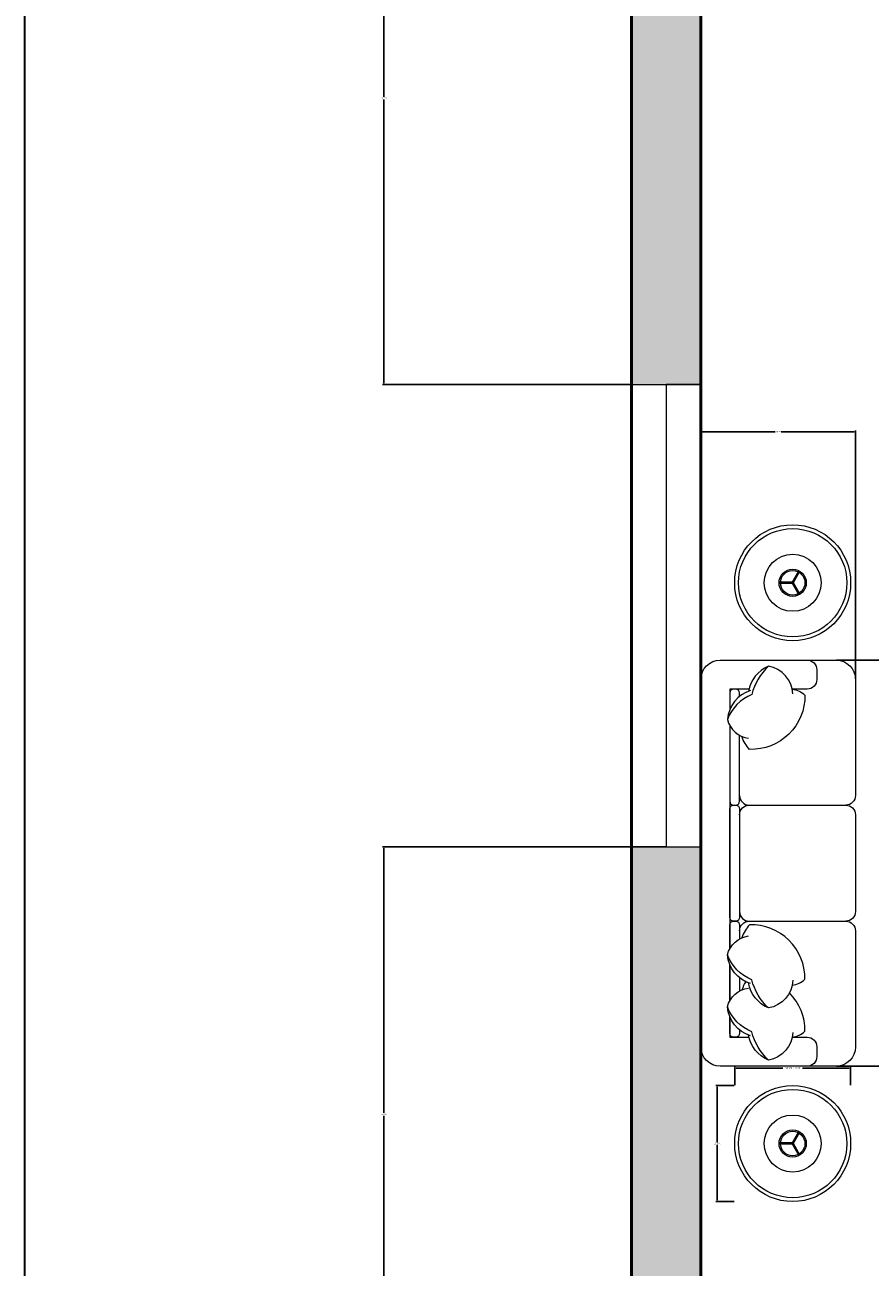
# Model space of a CAD drawing. Units: inches. Extents: x 1676 to 2199, y 1657 to 2783.
# Tile 2 of 10: x 1676 to 1786, y 1905 to 2066. Entities that reach past the tile are written whole.
import ezdxf

# ---------------------------------------------------------------- set-up
doc = ezdxf.new("R2010")
doc.units = ezdxf.units.IN
for name, color, linetype, lineweight in [('A-ANNO-DIMS', 2, 'Continuous', 18), ('A-ANNO-TTLB', 7, 'Continuous', 35), ('A-FURN', 8, 'Continuous', 13), ('A-GLAZ', 4, 'Continuous', 18), ('A-WALL', 7, 'Continuous', 50)]:
    doc.layers.add(name, color=color, linetype=linetype, lineweight=lineweight)
doc.layers.add('A-WALL-PATT', color=251, linetype='Continuous', lineweight=13, true_color=0x636466)
doc.styles.get("Standard").update_dxf_attribs({"font": 'arial.ttf'})
doc.dimstyles.get("Standard").update_dxf_attribs({"dimtxt": 0.18, "dimasz": 0.18, "dimexe": 0.18, "dimexo": 0.0625, "dimgap": 0.09, "dimtad": 0, "dimtih": 1, "dimtoh": 1, "dimdec": 4, "dimzin": 0, "dimdsep": 46, "dimtxsty": 'Standard', "dimcen": 0.09, "dimadec": 0, "dimazin": 0, "dimtfac": 1, "dimtdec": 4, "dimtofl": 0, "dimtmove": 0, "dimatfit": 3, "dimfxl": 1, "dimtolj": 1, "dimtzin": 0, "dimarcsym": 0})

# ---------------------------------------------------------------- blocks, each defined once
blk = doc.blocks.new('TABLE-END-ROUND')
at = {"ltscale": 0.03}
for p, q in [((0, 0.08), (-1.77, 0.08)), ((-0.07, 0.04), (0.82, 1.57)), ((0.07, -0.04), (0.95, 1.49)), ((0.07, 0.04), (0.95, -1.49)), ((0, -0.08), (-1.77, -0.08)), ((-0.07, -0.04), (0.82, -1.57))]:
    blk.add_line(p, q, dxfattribs=at)
for radius in [7.53, 3.7, 1.77, 1.59]:
    blk.add_circle((0, 0), radius, dxfattribs=at)
blk.add_circle((0, 0), 7.03)
blk = doc.blocks.new('WIN-60')
for p, q in [((0, 0), (9, 0)), ((9, 0), (4.5, 0)), ((4.5, 0), (4.5, -60)), ((4.5, -60), (0, -60)), ((0, -60), (9, -60))]:
    blk.add_line(p, q)
blk = doc.blocks.new('*D15')
at = {"layer": 'A-ANNO-DIMS', "color": 0, "lineweight": -2, "transparency": 16777216}
for p, q in [((1768.47, 1928.63), (1768.47, 1931.01)), ((1768.65, 1930.83), (1774.74, 1930.83)), ((1783.35, 1930.83), (1777.26, 1930.83)), ((1783.53, 1928.63), (1783.53, 1931.01))]:
    blk.add_line(p, q, dxfattribs=at)
at = {"layer": 'A-ANNO-DIMS', "color": 0, "transparency": 16777216}
for points in [[(1768.65, 1930.86), (1768.65, 1930.8), (1768.47, 1930.83)], [(1783.35, 1930.86), (1783.35, 1930.8), (1783.53, 1930.83)]]:
    blk.add_solid(points, dxfattribs=at)
at = {"layer": 'Defpoints', "color": 0, "transparency": 16777216}
for p in [(1783.53, 1930.83), (1768.47, 1928.57), (1783.53, 1928.57)]:
    blk.add_point(p, dxfattribs=at)
at = {"layer": 'A-ANNO-DIMS', "color": 0, "transparency": 16777216, "insert": (1776, 1930.83), "char_height": 0.18, "attachment_point": 5}
blk.add_mtext('\\A1;END TABLE 15 TYP.', dxfattribs=at)
blk = doc.blocks.new('*D16')
at = {"layer": 'A-ANNO-DIMS', "color": 0, "lineweight": -2, "transparency": 16777216}
for p, q in [((1768.41, 1928.57), (1766.03, 1928.57)), ((1766.21, 1928.39), (1766.21, 1921.22)), ((1766.21, 1913.68), (1766.21, 1920.85)), ((1768.41, 1913.5), (1766.03, 1913.5))]:
    blk.add_line(p, q, dxfattribs=at)
at = {"layer": 'A-ANNO-DIMS', "color": 0, "transparency": 16777216}
for points in [[(1766.18, 1928.39), (1766.24, 1928.39), (1766.21, 1928.57)], [(1766.18, 1913.68), (1766.24, 1913.68), (1766.21, 1913.5)]]:
    blk.add_solid(points, dxfattribs=at)
at = {"layer": 'Defpoints', "color": 0, "transparency": 16777216}
for p in [(1766.21, 1928.57), (1768.47, 1928.57), (1768.47, 1913.5)]:
    blk.add_point(p, dxfattribs=at)
at = {"layer": 'A-ANNO-DIMS', "color": 0, "transparency": 16777216, "insert": (1766.21, 1921.04), "char_height": 0.18, "attachment_point": 5}
blk.add_mtext('\\A1;15 TYP.', dxfattribs=at)
blk = doc.blocks.new('*D25')
at = {"layer": 'A-ANNO-DIMS', "color": 0, "lineweight": -2, "transparency": 16777216}
for p, q in [((1755.01, 1959.57), (1722.74, 1959.57)), ((1722.92, 1959.39), (1722.92, 1925.01)), ((1722.92, 1890.27), (1722.92, 1924.65)), ((1755.01, 1890.09), (1722.74, 1890.09))]:
    blk.add_line(p, q, dxfattribs=at)
at = {"layer": 'A-ANNO-DIMS', "color": 0, "transparency": 16777216}
for points in [[(1722.89, 1959.39), (1722.95, 1959.39), (1722.92, 1959.57)], [(1722.89, 1890.27), (1722.95, 1890.27), (1722.92, 1890.09)]]:
    blk.add_solid(points, dxfattribs=at)
at = {"layer": 'Defpoints', "color": 0, "transparency": 16777216}
for p in [(1722.92, 1959.57), (1755.07, 1959.57), (1755.07, 1890.09)]:
    blk.add_point(p, dxfattribs=at)
at = {"layer": 'A-ANNO-DIMS', "color": 0, "transparency": 16777216, "insert": (1722.92, 1924.83), "char_height": 0.18, "attachment_point": 5}
blk.add_mtext('\\A1;69.49', dxfattribs=at)
blk = doc.blocks.new('*D26')
at = {"layer": 'A-ANNO-DIMS', "color": 0, "lineweight": -2, "transparency": 16777216}
for p, q in [((1755.01, 2093.92), (1722.74, 2093.92)), ((1722.92, 2093.74), (1722.92, 2056.93)), ((1722.92, 2019.75), (1722.92, 2056.56)), ((1755.01, 2019.57), (1722.74, 2019.57))]:
    blk.add_line(p, q, dxfattribs=at)
at = {"layer": 'A-ANNO-DIMS', "color": 0, "transparency": 16777216}
for points in [[(1722.89, 2093.74), (1722.95, 2093.74), (1722.92, 2093.92)], [(1722.89, 2019.75), (1722.95, 2019.75), (1722.92, 2019.57)]]:
    blk.add_solid(points, dxfattribs=at)
at = {"layer": 'Defpoints', "color": 0, "transparency": 16777216}
for p in [(1722.92, 2093.92), (1755.07, 2093.92), (1755.07, 2019.57)]:
    blk.add_point(p, dxfattribs=at)
at = {"layer": 'A-ANNO-DIMS', "color": 0, "transparency": 16777216, "insert": (1722.92, 2056.75), "char_height": 0.18, "attachment_point": 5}
blk.add_mtext('\\A1;74.35', dxfattribs=at)
blk = doc.blocks.new('*D56')
at = {"layer": 'A-ANNO-DIMS', "color": 0, "lineweight": -2, "transparency": 16777216}
for p, q in [((1781.71, 1983.79), (1813.98, 1983.79)), ((1813.8, 1983.61), (1813.8, 1957.62)), ((1813.8, 1931.26), (1813.8, 1957.25)), ((1781.71, 1931.08), (1813.98, 1931.08))]:
    blk.add_line(p, q, dxfattribs=at)
at = {"layer": 'A-ANNO-DIMS', "color": 0, "transparency": 16777216}
for points in [[(1813.77, 1983.61), (1813.83, 1983.61), (1813.8, 1983.79)], [(1813.77, 1931.26), (1813.83, 1931.26), (1813.8, 1931.08)]]:
    blk.add_solid(points, dxfattribs=at)
at = {"layer": 'Defpoints', "color": 0, "transparency": 16777216}
for p in [(1781.65, 1983.79), (1781.65, 1931.08), (1813.8, 1931.08)]:
    blk.add_point(p, dxfattribs=at)
at = {"layer": 'A-ANNO-DIMS', "color": 0, "transparency": 16777216, "insert": (1813.8, 1957.43), "char_height": 0.18, "attachment_point": 5}
blk.add_mtext('\\A1;52.72', dxfattribs=at)
blk = doc.blocks.new('*D57')
at = {"layer": 'A-ANNO-DIMS', "color": 0, "lineweight": -2, "transparency": 16777216}
for p, q in [((1764.07, 1981.34), (1764.07, 2013.61)), ((1764.25, 2013.43), (1773.72, 2013.43)), ((1783.98, 2013.43), (1774.51, 2013.43)), ((1784.16, 1981.34), (1784.16, 2013.61))]:
    blk.add_line(p, q, dxfattribs=at)
at = {"layer": 'A-ANNO-DIMS', "color": 0, "transparency": 16777216}
for points in [[(1764.25, 2013.46), (1764.25, 2013.4), (1764.07, 2013.43)], [(1783.98, 2013.46), (1783.98, 2013.4), (1784.16, 2013.43)]]:
    blk.add_solid(points, dxfattribs=at)
at = {"layer": 'Defpoints', "color": 0, "transparency": 16777216}
for p in [(1784.16, 2013.43), (1764.07, 1981.28), (1784.16, 1981.28)]:
    blk.add_point(p, dxfattribs=at)
at = {"layer": 'A-ANNO-DIMS', "color": 0, "transparency": 16777216, "insert": (1774.12, 2013.43), "char_height": 0.18, "attachment_point": 5}
blk.add_mtext('\\A1;20.08', dxfattribs=at)

msp = doc.modelspace()

# ---------------------------------------------------------------- hatches: boundary and pattern name
at = {"layer": 'A-WALL-PATT'}
h = msp.add_hatch(color=256, dxfattribs=at)
h.dxf.hatch_style = 1
h.paths.add_polyline_path([(1945.4216, 2336.5871), (1945.4216, 2341.0871), (1755.075, 2341.0871), (1755.075, 2323.0739), (1764.075, 2323.0739), (1764.075, 2332.0871), (1945.4216, 2332.0871)])
h.paths.add_polyline_path([(1764.075, 2299.0739), (1755.075, 2299.0739), (1755.075, 2266.2601), (1759.575, 2266.2601), (1764.075, 2266.2601)])
h.paths.add_polyline_path([(1843.075, 2285.0871), (1764.075, 2285.0871), (1764.075, 2276.0871), (1843.075, 2276.0871)])
h.paths.add_polyline_path([(1931.075, 2332.0871), (1922.075, 2332.0871), (1922.075, 2285.0871), (1907.247, 2285.0871), (1907.247, 2276.0871), (1922.075, 2276.0871), (1922.075, 2263.0871), (1922.075, 2214.434), (1922.075, 2183.2198), (1931.075, 2183.2198), (1931.075, 2214.434), (1931.075, 2227.0871), (1991.075, 2227.0871), (1991.075, 2176.0871), (1991.075, 2167.0871), (2000.075, 2167.0871), (2133.075, 2167.0871), (2133.075, 2176.0871), (2000.075, 2176.0871), (2000.075, 2245.3418), (1995.575, 2245.3418), (1991.075, 2245.3418), (1991.075, 2236.0871), (1931.075, 2236.0871)])
h.paths.add_polyline_path([(2000.075, 2332.0871), (1991.075, 2332.0871), (1991.075, 2285.0871), (1991.075, 2274.6339), (2000.075, 2274.6339), (2000.075, 2285.0871)], flags=17)
h.paths.add_polyline_path([(2142.075, 2341.0871), (1969.4216, 2341.0871), (1969.4216, 2332.0871), (2133.075, 2332.0871), (2133.075, 2298.2101), (2142.075, 2298.2101)])
h.paths.add_polyline_path([(2142.075, 1844.9908), (2133.075, 1844.9908), (2133.075, 1790.0871), (2061.2106, 1790.0871), (2061.2106, 1781.0871), (2142.075, 1781.0871)])
h.paths.add_polyline_path([(2001.2106, 1790.0871), (1966.075, 1790.0871), (1966.075, 1957.0871), (1973.4183, 1957.0871), (1973.4183, 1966.0871), (1966.075, 1966.0871), (1966.075, 1983.1515), (1957.075, 1983.1515), (1957.075, 1899.0871), (1946.8789, 1899.0871), (1946.8789, 1890.0871), (1957.075, 1890.0871), (1957.075, 1781.0871), (2001.2106, 1781.0871), (2001.2106, 1785.5871)])
h.paths.add_polyline_path([(1876.3163, 1894.5871), (1876.3163, 1899.0871), (1820.9237, 1899.0871), (1820.9237, 1890.0871), (1876.3163, 1890.0871)])
h.paths.add_polyline_path([(1764.075, 2093.9207), (1759.575, 2093.9207), (1755.075, 2093.9207), (1755.075, 2019.5723), (1764.075, 2019.5723)])
h.paths.add_polyline_path([(1878.3926, 2083.0871), (1764.075, 2083.0871), (1764.075, 2074.0871), (1878.3926, 2074.0871)])
h.paths.add_polyline_path([(1764.075, 1959.5723), (1755.075, 1959.5723), (1755.075, 1890.0871), (1784.9237, 1890.0871), (1784.9237, 1894.5871), (1784.9237, 1899.0871), (1764.075, 1899.0871)])
h.paths.add_polyline_path([(2133.075, 2047.0871), (2000.075, 2047.0871), (1966.075, 2047.0871), (1957.075, 2047.0871), (1938.4046, 2047.0871), (1938.4046, 2038.0871), (1957.075, 2038.0871), (1957.075, 2026.1604), (1966.075, 2026.1604), (1966.075, 2038.0871), (2039.075, 2038.0871), (2039.075, 2011.4216), (2048.075, 2011.4216), (2048.075, 2038.0871), (2133.075, 2038.0871)])
h.paths.add_polyline_path([(2133.075, 1966.0871), (2048.075, 1966.0871), (2048.075, 1972.5045), (2039.075, 1972.5045), (2039.075, 1966.0871), (2025.1075, 1966.0871), (2025.1075, 1957.0871), (2133.075, 1957.0871)])
h.paths.add_polyline_path([(1764.075, 2206.2601), (1755.075, 2206.2601), (1755.075, 2153.9207), (1764.075, 2153.9207)])

# ---------------------------------------------------------------- linework, layer by layer
at = {"layer": 'A-ANNO-TTLB'}
msp.add_lwpolyline([(1676.2722, 2782.5054), (2199.4461, 2782.5054), (2199.4461, 1657.2705), (1676.2722, 1657.2705)], close=True, dxfattribs=at)
at = {"layer": 'A-FURN', "ltscale": 0.03}
msp.add_lwpolyline([(1781.6467, 1983.7912, -0.41421356), (1784.1569, 1981.2809), (1784.1569, 1966.2195, -0.41421356), (1782.9018, 1964.9643, -0.41421356), (1784.1569, 1963.7092), (1784.1569, 1951.158, -0.41421356), (1782.9018, 1949.9029, -0.41421356), (1784.1569, 1948.6478), (1784.1569, 1933.5863, -0.41421356), (1781.6467, 1931.0761), (1766.5852, 1931.0761, -0.41421356), (1764.075, 1933.5863), (1764.075, 1981.2809, -0.41421356), (1766.5852, 1983.7912)], format="xyb", close=True, dxfattribs=at)
at = {"layer": 'A-FURN'}
for points in [[(1777.8813, 1983.7912, -0.41421356), (1779.1364, 1982.536), (1779.1364, 1981.2809, -0.41421356), (1777.8813, 1980.0258), (1775.9367, 1980.0258)], [(1772.849, 1982.9924, 0.14772988), (1770.6919, 1979.324, 0.21334276), (1767.5282, 1976.0872, 0.17866181)], [(1776.0126, 1979.3959, 0.35677236), (1772.849, 1982.9924, 0.24954205), (1770.2418, 1979.7337, -9.61688035)], [(1770.52, 1979.8308, 0.30666349), (1767.5282, 1976.0872, 0.30632997), (1770.2605, 1973.6416, -0.87284716)], [(1769.0955, 1979.068), (1769.0955, 1979.5237, 0.41421356), (1768.5934, 1980.0258), (1768.3424, 1980.0258, 0.41421356), (1767.8403, 1979.5237)], [(1767.8403, 1979.5237), (1767.8403, 1977.3854, 0.41421356)], [(1775.9361, 1980.0285, -0.16554063), (1777.5945, 1979.2521, -0.42598917), (1770.4043, 1972.2031, -0.12152332), (1769.4133, 1973.8764, 7.11546429)], [(1767.8403, 1975.2973), (1767.8403, 1965.4664, 0.41421356), (1768.3424, 1964.9643), (1768.5934, 1964.9643, 0.41421356), (1769.0955, 1965.4664), (1769.0955, 1974.0335, 0.41421356)], [(1769.0955, 1966.2195, 0.41421356), (1770.3506, 1964.9643), (1782.9018, 1964.9643, 0.41421356)], [(1769.0955, 1963.7092, -0.41421356), (1770.3506, 1964.9643)], [(1767.8403, 1946.3312), (1767.8403, 1949.4008, -0.41421356), (1768.3424, 1949.9029), (1768.5934, 1949.9029, -0.41421356), (1769.0955, 1949.4008), (1769.0955, 1947.5951, -0.41421356)], [(1769.0955, 1951.158, 0.41421356), (1770.3506, 1949.9029)], [(1769.0955, 1948.6478, -0.41421356), (1770.3506, 1949.9029), (1782.9018, 1949.9029, -0.41421356)], [(1775.9361, 1941.6, 0.16554063), (1777.5945, 1942.3765, 0.42598917), (1770.4043, 1949.4255, 0.12152332), (1769.4133, 1947.7522, -7.11546429)], [(1770.52, 1941.7977, -0.30666349), (1767.5282, 1945.5413, -0.30632997), (1770.2605, 1947.9869, 0.87284716)], [(1772.849, 1938.6362, -0.14772988), (1770.6919, 1942.3045, -0.21334276), (1767.5282, 1945.5413, -0.17866181)], [(1767.8403, 1939.5699), (1767.8403, 1944.2432, -0.41421356)], [(1769.0955, 1942.5605), (1769.0955, 1940.8338, -0.41421356)], [(1769.9039, 1942.0431, 0.07186538), (1769.4133, 1940.9909, -7.11546429)], [(1776.0126, 1942.2326, -0.35677236), (1772.849, 1938.6362, -0.24954205), (1770.2418, 1941.8949, 9.61688035)], [(1770.52, 1935.0365, -0.30666349), (1767.5282, 1938.78, -0.30632997), (1770.2605, 1941.2256, 0.87284716)], [(1775.9361, 1934.8387, 0.16554063), (1777.5945, 1935.6152, 0.20023115), (1775.5747, 1940.5975, 0.12152332)], [(1772.849, 1931.8749, -0.14772988), (1770.6919, 1935.5432, -0.21334276), (1767.5282, 1938.78, -0.17866181)], [(1767.8403, 1937.4819), (1767.8403, 1934.8414), (1770.307, 1934.8414, -0.41421356)], [(1767.8403, 1935.3435), (1767.8403, 1937.4819, -0.41421356)], [(1769.0955, 1935.7992), (1769.0955, 1935.3435, -0.41421356), (1768.5934, 1934.8414), (1768.3424, 1934.8414, -0.41421356), (1767.8403, 1935.3435)], [(1776.0126, 1935.4713, -0.35677236), (1772.849, 1931.8749, -0.24954205), (1770.2418, 1935.1336, 9.61688035)], [(1775.9367, 1934.8414), (1777.8813, 1934.8414, -0.41421356), (1779.1364, 1933.5863), (1779.1364, 1932.3312, -0.41421356), (1777.8813, 1931.0761)]]:
    msp.add_lwpolyline(points, format="xyb", dxfattribs=at)
for points in [[(1770.307, 1980.0258), (1767.8403, 1980.0258), (1767.8403, 1977.3854)], [(1767.8403, 1975.2973), (1767.8403, 1946.3312)], [(1767.8403, 1944.2432), (1767.8403, 1939.5699)]]:
    msp.add_lwpolyline(points, dxfattribs=at)
msp.add_lwpolyline([(1767.8403, 1950.4049), (1767.8403, 1964.4623, -0.41421356), (1768.3424, 1964.9643), (1768.5934, 1964.9643, -0.41421356), (1769.0955, 1964.4623), (1769.0955, 1950.4049, -0.41421356), (1768.5934, 1949.9029), (1768.3424, 1949.9029, -0.41421356)], format="xyb", close=True, dxfattribs=at)
at = {"layer": 'A-WALL'}
for p, q in [((1755.075, 2341.0871), (1755.075, 1890.0871)), ((1764.075, 2332.0871), (1764.075, 1899.0871))]:
    msp.add_line(p, q, dxfattribs=at)

# ---------------------------------------------------------------- block references
at = {"layer": 'A-FURN'}
for p in [(1775.9986, 1993.8321), (1775.9986, 1921.0351)]:
    msp.add_blockref('TABLE-END-ROUND', p, dxfattribs=at)
at = {"layer": 'A-GLAZ'}
msp.add_blockref('WIN-60', (1755.075, 2019.5723), dxfattribs=at)

# ---------------------------------------------------------------- dimensions: what is measured, and where the dimension line sits
at = {"layer": 'A-ANNO-DIMS'}
for base, p1, p2, angle, picture, middle in [((1722.925, 2093.9207), (1755.075, 2019.5723), (1755.075, 2093.9207), 90, '*D26', (1722.925, 2056.7465)), ((1813.7967, 1931.0761), (1781.6467, 1983.7912), (1781.6467, 1931.0761), 270, '*D56', (1813.7967, 1957.4336)), ((1722.925, 1959.5723), (1755.075, 1890.0871), (1755.075, 1959.5723), 90, '*D25', (1722.925, 1924.8297))]:
    dim = msp.add_linear_dim(base=base, p1=p1, p2=p2, angle=angle, dimstyle='Standard', override={"dimdec": 2, "dimlfac": 1, "dimrnd": 0, "dimzin": 0, "dimdsep": 46, "dimlunit": 2}, dxfattribs=at)
    dim.commit()
    dim.dimension.update_dxf_attribs({"geometry": picture, "text_midpoint": middle})
dim = msp.add_linear_dim(base=(1784.1569, 2013.4309), p1=(1764.075, 1981.2809), p2=(1784.1569, 1981.2809), dimstyle='Standard', override={"dimdec": 2, "dimlfac": 1, "dimrnd": 0, "dimzin": 0, "dimdsep": 46, "dimlunit": 2}, dxfattribs=at)
dim.commit()
dim.dimension.update_dxf_attribs({"geometry": '*D57', "text_midpoint": (1774.1159, 2013.4309)})
dim = msp.add_linear_dim(base=(1783.5294, 1930.8251), p1=(1768.4679, 1928.5658), p2=(1783.5294, 1928.5658), text='END TABLE <> TYP.', dimstyle='Standard', override={"dimdec": 0, "dimlfac": 1, "dimrnd": 0, "dimzin": 0, "dimdsep": 46, "dimlunit": 2}, dxfattribs=at)
dim.commit()
dim.dimension.update_dxf_attribs({"geometry": '*D15', "text_midpoint": (1775.9986, 1930.8251)})
dim = msp.add_linear_dim(base=(1766.2087, 1928.5658), p1=(1768.4679, 1913.5044), p2=(1768.4679, 1928.5658), angle=90, text='<> TYP.', dimstyle='Standard', override={"dimdec": 0, "dimlfac": 1, "dimrnd": 0, "dimzin": 0, "dimdsep": 46, "dimlunit": 2}, dxfattribs=at)
dim.commit()
dim.dimension.update_dxf_attribs({"geometry": '*D16', "text_midpoint": (1766.2087, 1921.0351)})

doc.saveas('drawing.dxf')
